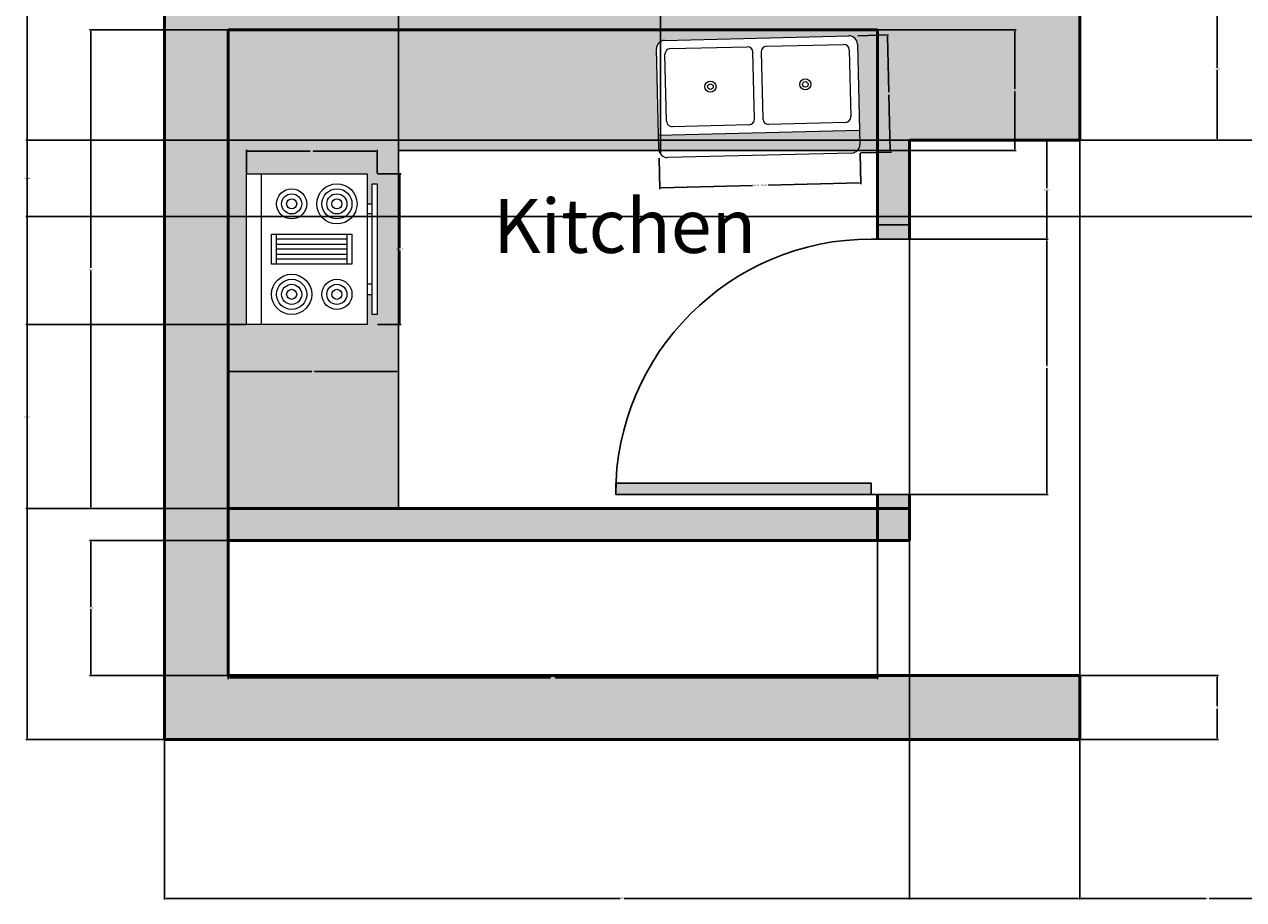
# Model space of a CAD drawing. Units: inches. Extents: x 2578 to 2919, y 51 to 451.
# Tile 1 of 5: x 2578 to 2750, y 51 to 174. Entities that reach past the tile are written whole.
import ezdxf

# ---------------------------------------------------------------- set-up
doc = ezdxf.new("R2010")
doc.units = ezdxf.units.IN
for name, color, linetype, lineweight in [('A-ANNO-DIMS', 2, 'Continuous', 18), ('A-AREA-IDEN', 7, 'Continuous', 25), ('A-DOOR', 4, 'Continuous', 25), ('A-EQPM', 8, 'Continuous', 18), ('A-FLOR-CASE', 8, 'Continuous', 25), ('A-FLOR-FIXT', 9, 'Continuous', 18), ('A-WALL', 7, 'Continuous', 50), ('A-WALL-PATT', 250, 'Continuous', 13)]:
    doc.layers.add(name, color=color, linetype=linetype, lineweight=lineweight)
doc.layers.add('A-CASE-PATT', color=9, linetype='Continuous', lineweight=13, true_color=0xc7c8ca)
doc.layers.add('A-DOOR-PATT', color=29, linetype='Continuous', lineweight=13, true_color=0x4f342a)
doc.styles.get("Standard").update_dxf_attribs({"font": 'arial.ttf'})
doc.dimstyles.get("Standard").update_dxf_attribs({"dimtxt": 0.18, "dimasz": 0.18, "dimexe": 0.18, "dimexo": 0.0625, "dimgap": 0.09, "dimtad": 0, "dimtih": 1, "dimtoh": 1, "dimdec": 4, "dimzin": 0, "dimdsep": 46, "dimtxsty": 'Standard', "dimcen": 0.09, "dimadec": 0, "dimazin": 0, "dimtfac": 1, "dimtdec": 4, "dimtofl": 0, "dimtmove": 0, "dimatfit": 3, "dimfxl": 1, "dimtolj": 1, "dimtzin": 0, "dimarcsym": 0})

# ---------------------------------------------------------------- blocks, each defined once
blk = doc.blocks.new('*U3')
for p, q in [((0, 0), (0, -6)), ((40, 0), (40, -6))]:
    blk.add_line(p, q)
blk.add_lwpolyline([(0, 0), (0, 40), (1.75, 40), (1.75, 0)], close=True)
blk.add_arc((0, 0), 40, 0, 90)
blk = doc.blocks.new('Range-Oven - 30 in top')
for p, q in [((0, -3), (30, -3)), ((12, -6), (18, -6)), ((13, -20), (13, -6)), ((14, -6), (14, -20)), ((15, -20), (15, -6)), ((16, -6), (16, -20)), ((17, -20), (17, -6)), ((18, -20), (12, -20)), ((6, -24), (6, -25)), ((8, -25), (8, -24)), ((22, -25), (22, -24)), ((24, -24), (24, -25))]:
    blk.add_line(p, q)
for points in [[(0, -24), (0, 0), (30, 0), (30, -24)], [(12, -21), (12, -5), (18, -5), (18, -21)], [(2, -26), (2, -25), (28, -25), (28, -26)]]:
    blk.add_lwpolyline(points, close=True)
for centre, radius in [((6, -9), 4), ((6, -9), 3), ((6, -9), 2), ((24, -9), 3), ((24, -9), 2), ((6, -9), 1), ((24, -9), 1), ((24, -18), 4), ((6, -18), 3), ((6, -18), 2), ((24, -18), 3), ((24, -18), 2), ((6, -18), 1), ((24, -18), 1)]:
    blk.add_circle(centre, radius)
blk = doc.blocks.new('Sink-double - 36 in top')
for p, q in [((-18, -4), (18, -4)), ((-0.75, -18.5), (-0.75, -6.5)), ((0.75, -6.5), (0.75, -18.5))]:
    blk.add_line(p, q)
for points in [[(-16.5, 0), (16.5, 0)], [(-18, -19.5), (-18, -1.5)], [(18, -1.5), (18, -19.5)], [(-16.5, -18.5), (-16.5, -6.5)], [(-15.5, -5.5), (-1.75, -5.5)], [(1.75, -5.5), (15.5, -5.5)], [(16.5, -6.5), (16.5, -18.5)], [(-1.75, -19.5), (-15.5, -19.5)], [(15.5, -19.5), (1.75, -19.5)], [(16.5, -21), (-16.5, -21)]]:
    blk.add_lwpolyline(points)
for centre, radius in [((-8.5, -12.5), 1), ((-8.5, -12.5), 0.5), ((8.5, -12.5), 1), ((8.5, -12.5), 0.5)]:
    blk.add_circle(centre, radius)
for centre, radius, start, end in [((-16.5, -1.5), 1.5, 90, 180), ((16.5, -1.5), 1.5, 0, 90), ((-15.5, -6.5), 1, 90, 180), ((-1.75, -6.5), 1, 0, 90), ((1.75, -6.5), 1, 90, 180), ((15.5, -6.5), 1, 0, 90), ((-16.5, -19.5), 1.5, 180, 270), ((-15.5, -18.5), 1, 180, 270), ((-1.75, -18.5), 1, 270, 0), ((1.75, -18.5), 1, 180, 270), ((15.5, -18.5), 1, 270, 0), ((16.5, -19.5), 1.5, 270, 0)]:
    blk.add_arc(centre, radius, start, end)
blk = doc.blocks.new('*D31')
at = {"layer": 'A-ANNO-DIMS', "color": 0, "lineweight": -2, "transparency": 16777216}
for p, q in [((2627.59, 152.86), (2630.9, 152.86)), ((2630.72, 152.68), (2630.72, 142.41)), ((2630.72, 131.78), (2630.72, 142.04)), ((2627.59, 131.6), (2630.9, 131.6))]:
    blk.add_line(p, q, dxfattribs=at)
at = {"layer": 'A-ANNO-DIMS', "color": 0, "transparency": 16777216}
for points in [[(2630.69, 152.68), (2630.75, 152.68), (2630.72, 152.86)], [(2630.69, 131.78), (2630.75, 131.78), (2630.72, 131.6)]]:
    blk.add_solid(points, dxfattribs=at)
at = {"layer": 'Defpoints', "color": 0, "transparency": 16777216}
for p in [(2627.53, 152.86), (2630.72, 152.86), (2627.53, 131.6)]:
    blk.add_point(p, dxfattribs=at)
at = {"layer": 'A-ANNO-DIMS', "color": 0, "transparency": 16777216, "insert": (2630.72, 142.23), "char_height": 0.18, "attachment_point": 5}
blk.add_mtext('\\A1;RANGE 21', dxfattribs=at)
blk = doc.blocks.new('*D32')
at = {"layer": 'A-ANNO-DIMS', "color": 0, "lineweight": -2, "transparency": 16777216}
for p, q in [((2609.1, 152.92), (2609.1, 156.22)), ((2609.28, 156.04), (2618.1, 156.04)), ((2627.35, 156.04), (2618.53, 156.04)), ((2627.53, 152.92), (2627.53, 156.22))]:
    blk.add_line(p, q, dxfattribs=at)
at = {"layer": 'A-ANNO-DIMS', "color": 0, "transparency": 16777216}
for points in [[(2609.28, 156.07), (2609.28, 156.01), (2609.1, 156.04)], [(2627.35, 156.07), (2627.35, 156.01), (2627.53, 156.04)]]:
    blk.add_solid(points, dxfattribs=at)
at = {"layer": 'Defpoints', "color": 0, "transparency": 16777216}
for p in [(2609.1, 156.04), (2609.1, 152.86), (2627.53, 152.86)]:
    blk.add_point(p, dxfattribs=at)
at = {"layer": 'A-ANNO-DIMS', "color": 0, "transparency": 16777216, "insert": (2618.32, 156.04), "char_height": 0.18, "attachment_point": 5}
blk.add_mtext('\\A1;18', dxfattribs=at)
blk = doc.blocks.new('*D33')
at = {"layer": 'A-ANNO-DIMS', "color": 0, "lineweight": -2, "transparency": 16777216}
for p, q in [((2667.26, 155.05), (2667.37, 150.69)), ((2695.58, 155.74), (2695.69, 151.38)), ((2667.54, 150.87), (2680.43, 151.18)), ((2695.5, 151.55), (2682.62, 151.24))]:
    blk.add_line(p, q, dxfattribs=at)
at = {"layer": 'A-ANNO-DIMS', "color": 0, "transparency": 16777216}
for points in [[(2695.5, 151.58), (2695.5, 151.52), (2695.68, 151.56)], [(2667.54, 150.9), (2667.54, 150.84), (2667.36, 150.87)]]:
    blk.add_solid(points, dxfattribs=at)
at = {"layer": 'Defpoints', "color": 0, "transparency": 16777216}
for p in [(2667.26, 155.11), (2695.58, 155.8), (2667.36, 150.87)]:
    blk.add_point(p, dxfattribs=at)
at = {"layer": 'A-ANNO-DIMS', "color": 0, "transparency": 16777216, "insert": (2681.52, 151.21), "char_height": 0.18, "attachment_point": 5}
blk.add_mtext('\\A1;DOUBLE SINK 28', dxfattribs=at)
blk = doc.blocks.new('*D34')
at = {"layer": 'A-ANNO-DIMS', "color": 0, "lineweight": -2, "transparency": 16777216}
for p, q in [((2695.24, 172.32), (2699.6, 172.43)), ((2699.43, 172.25), (2699.62, 164.35)), ((2699.82, 156.09), (2699.63, 163.99)), ((2695.64, 155.8), (2700.01, 155.91))]:
    blk.add_line(p, q, dxfattribs=at)
at = {"layer": 'A-ANNO-DIMS', "color": 0, "transparency": 16777216}
for points in [[(2699.46, 172.25), (2699.4, 172.25), (2699.42, 172.43)], [(2699.85, 156.09), (2699.79, 156.09), (2699.83, 155.91)]]:
    blk.add_solid(points, dxfattribs=at)
at = {"layer": 'Defpoints', "color": 0, "transparency": 16777216}
for p in [(2695.18, 172.32), (2695.58, 155.8), (2699.83, 155.91)]:
    blk.add_point(p, dxfattribs=at)
at = {"layer": 'A-ANNO-DIMS', "color": 0, "transparency": 16777216, "insert": (2699.62, 164.17), "char_height": 0.18, "attachment_point": 5}
blk.add_mtext('\\A1;17', dxfattribs=at)
blk = doc.blocks.new('*D36')
at = {"layer": 'A-ANNO-DIMS', "color": 0, "lineweight": -2, "transparency": 16777216}
for p, q in [((2597.48, 431.14), (2578.02, 431.14)), ((2578.2, 430.96), (2578.2, 252.3)), ((2578.2, 73.28), (2578.2, 251.94)), ((2597.48, 73.1), (2578.02, 73.1))]:
    blk.add_line(p, q, dxfattribs=at)
at = {"layer": 'A-ANNO-DIMS', "color": 0, "transparency": 16777216}
for points in [[(2578.17, 430.96), (2578.23, 430.96), (2578.2, 431.14)], [(2578.17, 73.28), (2578.23, 73.28), (2578.2, 73.1)]]:
    blk.add_solid(points, dxfattribs=at)
at = {"layer": 'Defpoints', "color": 0, "transparency": 16777216}
for p in [(2578.2, 431.14), (2597.55, 431.14), (2597.55, 73.1)]:
    blk.add_point(p, dxfattribs=at)
at = {"layer": 'A-ANNO-DIMS', "color": 0, "transparency": 16777216, "insert": (2578.2, 252.12), "char_height": 0.18, "attachment_point": 5}
blk.add_mtext('\\A1;358.04', dxfattribs=at)
blk = doc.blocks.new('*D43')
at = {"layer": 'A-ANNO-DIMS', "color": 0, "lineweight": -2, "transparency": 16777216}
for p, q in [((2606.48, 173.14), (2587.02, 173.14)), ((2587.2, 172.96), (2587.2, 139.57)), ((2587.2, 105.82), (2587.2, 139.21)), ((2606.48, 105.64), (2587.02, 105.64))]:
    blk.add_line(p, q, dxfattribs=at)
at = {"layer": 'A-ANNO-DIMS', "color": 0, "transparency": 16777216}
for points in [[(2587.17, 172.96), (2587.23, 172.96), (2587.2, 173.14)], [(2587.17, 105.82), (2587.23, 105.82), (2587.2, 105.64)]]:
    blk.add_solid(points, dxfattribs=at)
at = {"layer": 'Defpoints', "color": 0, "transparency": 16777216}
for p in [(2587.2, 173.14), (2606.55, 173.14), (2606.55, 105.64)]:
    blk.add_point(p, dxfattribs=at)
at = {"layer": 'A-ANNO-DIMS', "color": 0, "transparency": 16777216, "insert": (2587.2, 139.39), "char_height": 0.18, "attachment_point": 5}
blk.add_mtext('\\A1;67.5', dxfattribs=at)
blk = doc.blocks.new('*D44')
at = {"layer": 'A-ANNO-DIMS', "color": 0, "lineweight": -2, "transparency": 16777216}
for p, q in [((2606.48, 101.14), (2587.02, 101.14)), ((2587.2, 100.96), (2587.2, 91.8)), ((2587.2, 82.28), (2587.2, 91.44)), ((2606.48, 82.1), (2587.02, 82.1))]:
    blk.add_line(p, q, dxfattribs=at)
at = {"layer": 'A-ANNO-DIMS', "color": 0, "transparency": 16777216}
for points in [[(2587.17, 100.96), (2587.23, 100.96), (2587.2, 101.14)], [(2587.17, 82.28), (2587.23, 82.28), (2587.2, 82.1)]]:
    blk.add_solid(points, dxfattribs=at)
at = {"layer": 'Defpoints', "color": 0, "transparency": 16777216}
for p in [(2587.2, 101.14), (2606.55, 101.14), (2606.55, 82.1)]:
    blk.add_point(p, dxfattribs=at)
at = {"layer": 'A-ANNO-DIMS', "color": 0, "transparency": 16777216, "insert": (2587.2, 91.62), "char_height": 0.18, "attachment_point": 5}
blk.add_mtext('\\A1;19.04', dxfattribs=at)
blk = doc.blocks.new('*D45')
at = {"layer": 'A-ANNO-DIMS', "color": 0, "lineweight": -2, "transparency": 16777216}
for p, q in [((2606.55, 101.08), (2606.55, 81.61)), ((2698.05, 101.08), (2698.05, 81.61)), ((2606.73, 81.79), (2651.97, 81.79)), ((2697.87, 81.79), (2652.62, 81.79))]:
    blk.add_line(p, q, dxfattribs=at)
at = {"layer": 'A-ANNO-DIMS', "color": 0, "transparency": 16777216}
for points in [[(2606.73, 81.82), (2606.73, 81.76), (2606.55, 81.79)], [(2697.87, 81.82), (2697.87, 81.76), (2698.05, 81.79)]]:
    blk.add_solid(points, dxfattribs=at)
at = {"layer": 'Defpoints', "color": 0, "transparency": 16777216}
for p in [(2606.55, 101.14), (2698.05, 101.14), (2606.55, 81.79)]:
    blk.add_point(p, dxfattribs=at)
at = {"layer": 'A-ANNO-DIMS', "color": 0, "transparency": 16777216, "insert": (2652.3, 81.79), "char_height": 0.18, "attachment_point": 5}
blk.add_mtext('\\A1;91.5', dxfattribs=at)
blk = doc.blocks.new('*D50')
at = {"layer": 'A-ANNO-DIMS', "color": 0, "lineweight": -2, "transparency": 16777216}
for p, q in [((2597.55, 73.04), (2597.55, 50.5)), ((2726.55, 73.04), (2726.55, 50.5)), ((2597.73, 50.68), (2661.77, 50.68)), ((2726.37, 50.68), (2662.33, 50.68))]:
    blk.add_line(p, q, dxfattribs=at)
at = {"layer": 'A-ANNO-DIMS', "color": 0, "transparency": 16777216}
for points in [[(2597.73, 50.71), (2597.73, 50.65), (2597.55, 50.68)], [(2726.37, 50.71), (2726.37, 50.65), (2726.55, 50.68)]]:
    blk.add_solid(points, dxfattribs=at)
at = {"layer": 'Defpoints', "color": 0, "transparency": 16777216}
for p in [(2597.55, 73.1), (2726.55, 73.1), (2726.55, 50.68)]:
    blk.add_point(p, dxfattribs=at)
at = {"layer": 'A-ANNO-DIMS', "color": 0, "transparency": 16777216, "insert": (2662.05, 50.68), "char_height": 0.18, "attachment_point": 5}
blk.add_mtext('\\A1;129', dxfattribs=at)
blk = doc.blocks.new('*D51')
at = {"layer": 'A-ANNO-DIMS', "color": 0, "lineweight": -2, "transparency": 16777216}
for p, q in [((2726.55, 73.04), (2726.55, 50.5)), ((2762.55, 73.04), (2762.55, 50.5)), ((2726.73, 50.68), (2744.33, 50.68)), ((2762.37, 50.68), (2744.77, 50.68))]:
    blk.add_line(p, q, dxfattribs=at)
at = {"layer": 'A-ANNO-DIMS', "color": 0, "transparency": 16777216}
for points in [[(2726.73, 50.71), (2726.73, 50.65), (2726.55, 50.68)], [(2762.37, 50.71), (2762.37, 50.65), (2762.55, 50.68)]]:
    blk.add_solid(points, dxfattribs=at)
at = {"layer": 'Defpoints', "color": 0, "transparency": 16777216}
for p in [(2726.55, 73.1), (2762.55, 73.1), (2762.55, 50.68)]:
    blk.add_point(p, dxfattribs=at)
at = {"layer": 'A-ANNO-DIMS', "color": 0, "transparency": 16777216, "insert": (2744.55, 50.68), "char_height": 0.18, "attachment_point": 5}
blk.add_mtext('\\A1;36', dxfattribs=at)
blk = doc.blocks.new('*D56')
at = {"layer": 'A-ANNO-DIMS', "color": 0, "lineweight": -2, "transparency": 16777216}
for p, q in [((2702.61, 143.64), (2722.08, 143.64)), ((2721.9, 143.46), (2721.9, 125.82)), ((2721.9, 107.82), (2721.9, 125.46)), ((2702.61, 107.64), (2722.08, 107.64))]:
    blk.add_line(p, q, dxfattribs=at)
at = {"layer": 'A-ANNO-DIMS', "color": 0, "transparency": 16777216}
for points in [[(2721.87, 143.46), (2721.93, 143.46), (2721.9, 143.64)], [(2721.87, 107.82), (2721.93, 107.82), (2721.9, 107.64)]]:
    blk.add_solid(points, dxfattribs=at)
at = {"layer": 'Defpoints', "color": 0, "transparency": 16777216}
for p in [(2702.55, 143.64), (2702.55, 107.64), (2721.9, 107.64)]:
    blk.add_point(p, dxfattribs=at)
at = {"layer": 'A-ANNO-DIMS', "color": 0, "transparency": 16777216, "insert": (2721.9, 125.64), "char_height": 0.18, "attachment_point": 5}
blk.add_mtext('\\A1;36', dxfattribs=at)
blk = doc.blocks.new('*D59')
at = {"layer": 'A-ANNO-DIMS', "color": 0, "lineweight": -2, "transparency": 16777216}
for p, q in [((2702.61, 157.6), (2722.08, 157.6)), ((2721.9, 157.42), (2721.9, 150.8)), ((2721.9, 143.82), (2721.9, 150.44)), ((2702.61, 143.64), (2722.08, 143.64))]:
    blk.add_line(p, q, dxfattribs=at)
at = {"layer": 'A-ANNO-DIMS', "color": 0, "transparency": 16777216}
for points in [[(2721.87, 157.42), (2721.93, 157.42), (2721.9, 157.6)], [(2721.87, 143.82), (2721.93, 143.82), (2721.9, 143.64)]]:
    blk.add_solid(points, dxfattribs=at)
at = {"layer": 'Defpoints', "color": 0, "transparency": 16777216}
for p in [(2702.55, 157.6), (2702.55, 143.64), (2721.9, 143.64)]:
    blk.add_point(p, dxfattribs=at)
at = {"layer": 'A-ANNO-DIMS', "color": 0, "transparency": 16777216, "insert": (2721.9, 150.62), "char_height": 0.18, "attachment_point": 5}
blk.add_mtext('\\A1;13.958', dxfattribs=at)
blk = doc.blocks.new('*D60')
at = {"layer": 'A-ANNO-DIMS', "color": 0, "lineweight": -2, "transparency": 16777216}
for p, q in [((2726.61, 82.1), (2746.08, 82.1)), ((2745.9, 81.92), (2745.9, 77.78)), ((2745.9, 73.28), (2745.9, 77.42)), ((2726.61, 73.1), (2746.08, 73.1))]:
    blk.add_line(p, q, dxfattribs=at)
at = {"layer": 'A-ANNO-DIMS', "color": 0, "transparency": 16777216}
for points in [[(2745.87, 81.92), (2745.93, 81.92), (2745.9, 82.1)], [(2745.87, 73.28), (2745.93, 73.28), (2745.9, 73.1)]]:
    blk.add_solid(points, dxfattribs=at)
at = {"layer": 'Defpoints', "color": 0, "transparency": 16777216}
for p in [(2726.55, 82.1), (2726.55, 73.1), (2745.9, 73.1)]:
    blk.add_point(p, dxfattribs=at)
at = {"layer": 'A-ANNO-DIMS', "color": 0, "transparency": 16777216, "insert": (2745.9, 77.6), "char_height": 0.18, "attachment_point": 5}
blk.add_mtext('\\A1;9', dxfattribs=at)
blk = doc.blocks.new('*D62')
at = {"layer": 'A-ANNO-DIMS', "color": 0, "lineweight": -2, "transparency": 16777216}
for p, q in [((2606.55, 105.7), (2606.55, 125.17)), ((2606.73, 124.99), (2618.33, 124.99)), ((2630.37, 124.99), (2618.77, 124.99)), ((2630.55, 105.7), (2630.55, 125.17))]:
    blk.add_line(p, q, dxfattribs=at)
at = {"layer": 'A-ANNO-DIMS', "color": 0, "transparency": 16777216}
for points in [[(2606.73, 125.02), (2606.73, 124.96), (2606.55, 124.99)], [(2630.37, 125.02), (2630.37, 124.96), (2630.55, 124.99)]]:
    blk.add_solid(points, dxfattribs=at)
at = {"layer": 'Defpoints', "color": 0, "transparency": 16777216}
for p in [(2630.55, 124.99), (2606.55, 105.64), (2630.55, 105.64)]:
    blk.add_point(p, dxfattribs=at)
at = {"layer": 'A-ANNO-DIMS', "color": 0, "transparency": 16777216, "insert": (2618.55, 124.99), "char_height": 0.18, "attachment_point": 5}
blk.add_mtext('\\A1;24', dxfattribs=at)
blk = doc.blocks.new('*D63')
at = {"layer": 'A-ANNO-DIMS', "color": 0, "lineweight": -2, "transparency": 16777216}
for p, q in [((2698.11, 173.14), (2717.58, 173.14)), ((2717.4, 172.96), (2717.4, 164.82)), ((2717.4, 156.32), (2717.4, 164.46)), ((2698.11, 156.14), (2717.58, 156.14))]:
    blk.add_line(p, q, dxfattribs=at)
at = {"layer": 'A-ANNO-DIMS', "color": 0, "transparency": 16777216}
for points in [[(2717.37, 172.96), (2717.43, 172.96), (2717.4, 173.14)], [(2717.37, 156.32), (2717.43, 156.32), (2717.4, 156.14)]]:
    blk.add_solid(points, dxfattribs=at)
at = {"layer": 'Defpoints', "color": 0, "transparency": 16777216}
for p in [(2698.05, 173.14), (2698.05, 156.14), (2717.4, 156.14)]:
    blk.add_point(p, dxfattribs=at)
at = {"layer": 'A-ANNO-DIMS', "color": 0, "transparency": 16777216, "insert": (2717.4, 164.64), "char_height": 0.18, "attachment_point": 5}
blk.add_mtext('\\A1;17', dxfattribs=at)
blk = doc.blocks.new('*D64')
at = {"layer": 'A-ANNO-DIMS', "color": 0, "lineweight": -2, "transparency": 16777216}
for p, q in [((2702.55, 157.54), (2702.55, 50.5)), ((2726.55, 157.54), (2726.55, 50.5)), ((2702.73, 50.68), (2714.33, 50.68)), ((2726.37, 50.68), (2714.77, 50.68))]:
    blk.add_line(p, q, dxfattribs=at)
at = {"layer": 'A-ANNO-DIMS', "color": 0, "transparency": 16777216}
for points in [[(2702.73, 50.71), (2702.73, 50.65), (2702.55, 50.68)], [(2726.37, 50.71), (2726.37, 50.65), (2726.55, 50.68)]]:
    blk.add_solid(points, dxfattribs=at)
at = {"layer": 'Defpoints', "color": 0, "transparency": 16777216}
for p in [(2702.55, 157.6), (2726.55, 157.6), (2726.55, 50.68)]:
    blk.add_point(p, dxfattribs=at)
at = {"layer": 'A-ANNO-DIMS', "color": 0, "transparency": 16777216, "insert": (2714.55, 50.68), "char_height": 0.18, "attachment_point": 5}
blk.add_mtext('\\A1;24', dxfattribs=at)
blk = doc.blocks.new('*D65')
at = {"layer": 'A-ANNO-DIMS', "color": 0, "lineweight": -2, "transparency": 16777216}
for p, q in [((2726.61, 177.64), (2746.08, 177.64)), ((2745.9, 177.46), (2745.9, 167.8)), ((2745.9, 157.78), (2745.9, 167.44)), ((2726.61, 157.6), (2746.08, 157.6))]:
    blk.add_line(p, q, dxfattribs=at)
at = {"layer": 'A-ANNO-DIMS', "color": 0, "transparency": 16777216}
for points in [[(2745.87, 177.46), (2745.93, 177.46), (2745.9, 177.64)], [(2745.87, 157.78), (2745.93, 157.78), (2745.9, 157.6)]]:
    blk.add_solid(points, dxfattribs=at)
at = {"layer": 'Defpoints', "color": 0, "transparency": 16777216}
for p in [(2726.55, 177.64), (2726.55, 157.6), (2745.9, 157.6)]:
    blk.add_point(p, dxfattribs=at)
at = {"layer": 'A-ANNO-DIMS', "color": 0, "transparency": 16777216, "insert": (2745.9, 167.62), "char_height": 0.18, "attachment_point": 5}
blk.add_mtext('\\A1;20.04', dxfattribs=at)
blk = doc.blocks.new('*D67')
at = {"layer": 'A-ANNO-DIMS', "color": 0, "lineweight": -2, "transparency": 16777216}
for p, q in [((2829.12, 157.6), (2578.02, 157.6)), ((2578.2, 157.42), (2578.2, 152.39)), ((2578.2, 146.99), (2578.2, 152.02)), ((2841.13, 146.81), (2578.02, 146.81))]:
    blk.add_line(p, q, dxfattribs=at)
at = {"layer": 'A-ANNO-DIMS', "color": 0, "transparency": 16777216}
for points in [[(2578.17, 157.42), (2578.23, 157.42), (2578.2, 157.6)], [(2578.17, 146.99), (2578.23, 146.99), (2578.2, 146.81)]]:
    blk.add_solid(points, dxfattribs=at)
at = {"layer": 'Defpoints', "color": 0, "transparency": 16777216}
for p in [(2578.2, 157.6), (2829.18, 157.6), (2841.19, 146.81)]:
    blk.add_point(p, dxfattribs=at)
at = {"layer": 'A-ANNO-DIMS', "color": 0, "transparency": 16777216, "insert": (2578.2, 152.21), "char_height": 0.18, "attachment_point": 5}
blk.add_mtext('\\A1;10.788', dxfattribs=at)
blk = doc.blocks.new('*D69')
at = {"layer": 'A-ANNO-DIMS', "color": 0, "lineweight": -2, "transparency": 16777216}
for p, q in [((2609.04, 131.6), (2578.02, 131.6)), ((2578.2, 131.42), (2578.2, 118.8)), ((2578.2, 105.82), (2578.2, 118.44)), ((2606.48, 105.64), (2578.02, 105.64))]:
    blk.add_line(p, q, dxfattribs=at)
at = {"layer": 'A-ANNO-DIMS', "color": 0, "transparency": 16777216}
for points in [[(2578.17, 131.42), (2578.23, 131.42), (2578.2, 131.6)], [(2578.17, 105.82), (2578.23, 105.82), (2578.2, 105.64)]]:
    blk.add_solid(points, dxfattribs=at)
at = {"layer": 'Defpoints', "color": 0, "transparency": 16777216}
for p in [(2578.2, 131.6), (2609.1, 131.6), (2606.55, 105.64)]:
    blk.add_point(p, dxfattribs=at)
at = {"layer": 'A-ANNO-DIMS', "color": 0, "transparency": 16777216, "insert": (2578.2, 118.62), "char_height": 0.18, "attachment_point": 5}
blk.add_mtext('\\A1;25.955', dxfattribs=at)
blk = doc.blocks.new('*D70')
at = {"layer": 'A-ANNO-DIMS', "color": 0, "lineweight": -2, "transparency": 16777216}
for p, q in [((2630.55, 156.2), (2630.55, 450.67)), ((2630.73, 450.49), (2648.67, 450.49)), ((2667.27, 450.49), (2649.32, 450.49)), ((2667.45, 155.71), (2667.45, 450.67))]:
    blk.add_line(p, q, dxfattribs=at)
at = {"layer": 'A-ANNO-DIMS', "color": 0, "transparency": 16777216}
for points in [[(2630.73, 450.52), (2630.73, 450.46), (2630.55, 450.49)], [(2667.27, 450.52), (2667.27, 450.46), (2667.45, 450.49)]]:
    blk.add_solid(points, dxfattribs=at)
at = {"layer": 'Defpoints', "color": 0, "transparency": 16777216}
for p in [(2667.45, 450.49), (2630.55, 156.14), (2667.45, 155.64)]:
    blk.add_point(p, dxfattribs=at)
at = {"layer": 'A-ANNO-DIMS', "color": 0, "transparency": 16777216, "insert": (2649, 450.49), "char_height": 0.18, "attachment_point": 5}
blk.add_mtext('\\A1;36.9', dxfattribs=at)

msp = doc.modelspace()

# ---------------------------------------------------------------- hatches: boundary and pattern name
at = {"layer": 'A-CASE-PATT'}
h = msp.add_hatch(color=256, dxfattribs=at)
h.dxf.hatch_style = 1
h.paths.add_polyline_path([(2698.047, 173.1406), (2606.547, 173.1406), (2606.547, 105.6406), (2630.547, 105.6406), (2630.547, 156.1406), (2698.047, 156.1406)])
h.paths.add_polyline_path([(2666.8862, 170.4525, -0.41421356), (2668.0374, 171.6612), (2693.9958, 172.2937, -0.41421356), (2695.2045, 171.1425), (2695.5016, 158.9499), (2667.1833, 158.26)], flags=16)
h.paths.add_polyline_path([(2668.0853, 169.6947, -0.41421356), (2668.8528, 170.5005), (2679.6688, 170.764, -0.41421356), (2680.4746, 169.9965), (2680.7046, 160.5571, -0.41421356), (2679.9371, 159.7513), (2669.1211, 159.4878, -0.41421356), (2668.3153, 160.2553)], flags=0)
h.paths.add_polyline_path([(2627.5279, 151.4383), (2627.5279, 133.0127), (2626.8192, 133.0127), (2626.8192, 135.8474), (2626.1105, 135.8474), (2626.1105, 131.5954), (2609.1023, 131.5954), (2609.1023, 152.8557), (2626.1105, 152.8557), (2626.1105, 148.6036), (2626.8192, 148.6036), (2626.8192, 151.4383)], flags=16)
h.paths.add_polyline_path([(2675.2801, 165.1283, -1), (2673.7064, 165.1283, -1)], flags=0)
h.paths.add_polyline_path([(2674.8867, 165.1283, -1), (2674.0999, 165.1283, -1)], flags=0)
h.paths.add_polyline_path([(2624.6932, 148.6036, -1), (2619.0238, 148.6036, -1)], flags=0)
h.paths.add_polyline_path([(2623.9845, 148.6036, -1), (2619.7324, 148.6036, -1)], flags=0)
h.paths.add_polyline_path([(2623.2758, 148.6036, -1), (2620.4411, 148.6036, -1)], flags=0)
h.paths.add_polyline_path([(2622.5671, 148.6036, -1), (2621.1498, 148.6036, -1)], flags=0)
h.paths.add_polyline_path([(2623.9845, 144.3516), (2623.9845, 140.0995), (2612.6457, 140.0995), (2612.6457, 144.3516)], flags=0)
h.paths.add_polyline_path([(2623.2758, 140.8082), (2613.3543, 140.8082), (2613.3543, 143.6429), (2623.2758, 143.6429)], flags=0)
h.paths.add_polyline_path([(2617.6064, 148.6036, -1), (2613.3543, 148.6036, -1)], flags=0)
h.paths.add_polyline_path([(2681.6545, 170.0253, -0.41421356), (2682.422, 170.8311), (2693.238, 171.0946, -0.41421356), (2694.0437, 170.3271), (2694.2737, 160.8877, -0.41421356), (2693.5063, 160.0819), (2682.6903, 159.8184, -0.41421356), (2681.8845, 160.5859)], flags=0)
h.paths.add_polyline_path([(2616.8977, 148.6036, -1), (2614.063, 148.6036, -1)], flags=0)
h.paths.add_polyline_path([(2616.1891, 148.6036, -1), (2614.7717, 148.6036, -1)], flags=0)
h.paths.add_polyline_path([(2623.9845, 135.8474, -1), (2619.7324, 135.8474, -1)], flags=0)
h.paths.add_polyline_path([(2623.2758, 135.8474, -1), (2620.4411, 135.8474, -1)], flags=0)
h.paths.add_polyline_path([(2622.5671, 135.8474, -1), (2621.1498, 135.8474, -1)], flags=0)
h.paths.add_polyline_path([(2688.6526, 165.4541, -1), (2687.0789, 165.4541, -1)], flags=0)
h.paths.add_polyline_path([(2688.2592, 165.4541, -1), (2687.4724, 165.4541, -1)], flags=0)
h.paths.add_polyline_path([(2618.3151, 135.8474, -1), (2612.6457, 135.8474, -1)], flags=0)
h.paths.add_polyline_path([(2617.6064, 135.8474, -1), (2613.3543, 135.8474, -1)], flags=0)
h.paths.add_polyline_path([(2616.8977, 135.8474, -1), (2614.063, 135.8474, -1)], flags=0)
h.paths.add_polyline_path([(2616.1891, 135.8474, -1), (2614.7717, 135.8474, -1)], flags=0)
at = {"layer": 'A-DOOR-PATT'}
h = msp.add_hatch(color=256, dxfattribs=at)
h.dxf.hatch_style = 1
h.paths.add_polyline_path([(2717.5545, 331.5492, 0.01094143), (2715.9791, 331.5147), (2715.9791, 295.5417), (2717.5545, 295.5417)])
h.paths.add_polyline_path([(2772.7563, 343.5147, 0.01094143), (2771.181, 343.5492), (2771.181, 307.5417), (2772.7563, 307.5417)])
h.paths.add_polyline_path([(2809.181, 302.1406), (2807.181, 302.1406), (2807.181, 297.6406), (2809.181, 297.6406)])
h.paths.add_polyline_path([(2681.547, 290.1406), (2679.547, 290.1406), (2679.547, 285.6406), (2681.547, 285.6406)])
h.paths.add_polyline_path([(2870.5896, 193.5988), (2834.5821, 193.5988), (2834.5821, 192.0235), (2870.5551, 192.0235, 0.01094143)])
h.paths.add_polyline_path([(2829.181, 157.5988), (2824.681, 157.5988), (2824.681, 155.5988), (2829.181, 155.5988)])
h.paths.add_polyline_path([(2702.547, 145.6406), (2698.047, 145.6406), (2698.047, 143.6481), (2702.547, 143.6481)])
h.paths.add_polyline_path([(2697.1459, 109.2159), (2661.1384, 109.2159), (2661.1384, 107.6406), (2697.1459, 107.6406)])
h.paths.add_polyline_path([(2702.547, 107.6406), (2698.047, 107.6406), (2698.047, 105.6406), (2702.547, 105.6406)])
h.paths.add_polyline_path([(2771.181, 302.1406), (2769.181, 302.1406), (2769.181, 297.6406), (2771.181, 297.6406)])
at = {"layer": 'A-WALL-PATT'}
h = msp.add_hatch(color=256, dxfattribs=at)
h.dxf.hatch_style = 1
h.paths.add_polyline_path([(2606.547, 422.1406), (2889.181, 422.1406), (2889.181, 210.611), (2824.681, 210.611), (2824.681, 193.5988), (2829.181, 193.5988), (2829.181, 206.111), (2889.181, 206.111), (2889.181, 99.5988), (2829.181, 99.5988), (2829.181, 155.5988), (2824.681, 155.5988), (2824.681, 95.0988), (2889.181, 95.0988), (2889.181, 82.1022), (2762.547, 82.1022), (2762.547, 73.1022), (2898.181, 73.1022), (2898.181, 233.1022), (2898.181, 431.1406), (2597.547, 431.1406), (2597.547, 73.1022), (2726.547, 73.1022), (2726.547, 82.1022), (2606.547, 82.1022), (2606.547, 173.1406), (2698.047, 173.1406), (2698.047, 145.6406), (2702.547, 145.6406), (2702.547, 157.5988), (2726.547, 157.5988), (2726.547, 177.6406), (2606.547, 177.6406)])
h.paths.add_polyline_path([(2889.181, 302.1406), (2809.181, 302.1406), (2809.181, 297.6406), (2889.181, 297.6406)], flags=17)
h.paths.add_polyline_path([(2679.547, 290.1406), (2606.547, 290.1406), (2606.547, 285.6406), (2679.547, 285.6406)], flags=17)
h.paths.add_polyline_path([(2824.681, 157.5988), (2800.681, 157.5988), (2800.681, 155.5988), (2824.681, 155.5988)], flags=17)
h.paths.add_polyline_path([(2698.047, 105.6406), (2606.547, 105.6406), (2606.547, 101.1406), (2698.047, 101.1406)], flags=17)
h.paths.add_polyline_path([(2702.547, 105.6406), (2698.047, 105.6406), (2698.047, 101.1406), (2702.547, 101.1406)], flags=17)
h.paths.add_polyline_path([(2726.547, 422.1406), (2722.047, 422.1406), (2722.047, 295.5417), (2717.5545, 295.5417), (2717.5545, 290.1406), (2717.5504, 285.6406), (2722.047, 285.6406), (2726.547, 285.6406)], flags=17)
h.paths.add_polyline_path([(2769.181, 422.1406), (2764.681, 422.1406), (2764.681, 297.6406), (2769.181, 297.6406)], flags=17)

# ---------------------------------------------------------------- linework, layer by layer
at = {"layer": 'A-DOOR'}
for p, q in [((2698.047, 145.6406), (2702.547, 145.6406)), ((2698.047, 143.6406), (2702.547, 143.6406)), ((2698.047, 107.6406), (2702.547, 107.6406))]:
    msp.add_line(p, q, dxfattribs=at)
at = {"layer": 'A-FLOR-CASE'}
for p, q in [((2630.547, 105.6406), (2630.547, 156.1406)), ((2630.547, 156.1406), (2698.047, 156.1406))]:
    msp.add_line(p, q, dxfattribs=at)
at = {"layer": 'A-WALL'}
for p, q in [((2726.547, 157.5988), (2726.547, 177.6406)), ((2606.547, 82.1022), (2606.547, 173.1406)), ((2606.547, 173.1406), (2698.047, 173.1406)), ((2698.047, 143.6406), (2698.047, 173.1406)), ((2702.547, 143.6406), (2702.547, 157.5988)), ((2726.547, 157.5988), (2702.547, 157.5988)), ((2698.047, 101.1406), (2698.047, 107.6406)), ((2702.547, 101.1406), (2702.547, 107.6406)), ((2606.547, 105.6406), (2702.547, 105.6406)), ((2606.547, 101.1406), (2702.547, 101.1406)), ((2726.547, 82.1022), (2606.547, 82.1022)), ((2726.547, 73.1022), (2726.547, 82.1022))]:
    msp.add_line(p, q, dxfattribs=at)
msp.add_lwpolyline([(2726.547, 73.1022), (2597.547, 73.1022), (2597.547, 431.1406), (2898.181, 431.1406), (2898.181, 233.1022), (2898.181, 73.1022), (2762.547, 73.1022)], dxfattribs=at)

# ---------------------------------------------------------------- block references
at = {"layer": 'A-DOOR', "xscale": 0.9001866182309679, "yscale": 0.9001866182309679, "zscale": 0.9001866182309679, "rotation": 90}
msp.add_blockref('*U3', (2697.1459, 107.6406), dxfattribs=at)
at = {"layer": 'A-EQPM', "xscale": 0.7086762119144434, "yscale": 0.7086762119144434, "zscale": 0.7086762119144434, "rotation": 90}
msp.add_blockref('Range-Oven - 30 in top', (2609.1023, 131.5954), dxfattribs=at)
at = {"layer": 'A-FLOR-FIXT', "xscale": 0.7868516800692607, "yscale": 0.7868516800692607, "zscale": 0.7868516800692607, "rotation": 181.3956621728925}
msp.add_blockref('Sink-double - 36 in top', (2681.4191, 155.4585), dxfattribs=at)

# ---------------------------------------------------------------- texts
at = {"layer": 'A-AREA-IDEN'}
msp.add_text('Kitchen ', height=7.59312, dxfattribs=at).set_placement((2643.8829, 141.6902))

# ---------------------------------------------------------------- dimensions: what is measured, and where the dimension line sits
at = {"layer": 'A-ANNO-DIMS'}
for base, p1, p2, override, picture, middle in [((2667.4454, 450.4906), (2630.547, 156.1406), (2667.4454, 155.6436), {"dimdec": 1, "dimlfac": 1, "dimrnd": 0, "dimzin": 0, "dimdsep": 46, "dimlunit": 2}, '*D70', (2648.9962, 450.4906)), ((2726.547, 50.6838), (2702.547, 157.5988), (2726.547, 157.5988), {"dimdec": 0, "dimlfac": 1, "dimrnd": 0, "dimzin": 0, "dimdsep": 46, "dimlunit": 2}, '*D64', (2714.547, 50.6838)), ((2630.547, 124.9906), (2606.547, 105.6406), (2630.547, 105.6406), {"dimdec": 0, "dimlfac": 1, "dimrnd": 0, "dimzin": 0, "dimdsep": 46, "dimlunit": 2}, '*D62', (2618.547, 124.9906)), ((2726.547, 50.6838), (2597.547, 73.1022), (2726.547, 73.1022), {"dimdec": 0, "dimlfac": 1, "dimrnd": 0, "dimzin": 0, "dimdsep": 46, "dimlunit": 2}, '*D50', (2662.047, 50.6838)), ((2762.547, 50.6838), (2726.547, 73.1022), (2762.547, 73.1022), {"dimdec": 0, "dimlfac": 1, "dimrnd": 0, "dimzin": 0, "dimdsep": 46, "dimlunit": 2}, '*D51', (2744.547, 50.6838))]:
    dim = msp.add_linear_dim(base=base, p1=p1, p2=p2, dimstyle='Standard', override=override, dxfattribs=at)
    dim.commit()
    dim.dimension.update_dxf_attribs({"geometry": picture, "text_midpoint": middle})
for base, p1, p2, angle, override, picture, middle in [((2578.197, 431.1406), (2597.547, 73.1022), (2597.547, 431.1406), 90, {"dimdec": 2, "dimlfac": 1, "dimrnd": 0, "dimzin": 0, "dimdsep": 46, "dimlunit": 2}, '*D36', (2578.197, 252.1214)), ((2745.897, 157.5988), (2726.547, 177.6406), (2726.547, 157.5988), 270, {"dimdec": 2, "dimlfac": 1, "dimrnd": 0, "dimzin": 0, "dimdsep": 46, "dimlunit": 2}, '*D65', (2745.897, 167.6197)), ((2587.197, 173.1406), (2606.547, 105.6406), (2606.547, 173.1406), 90, {"dimdec": 1, "dimlfac": 1, "dimrnd": 0, "dimzin": 0, "dimdsep": 46, "dimlunit": 2}, '*D43', (2587.197, 139.3906)), ((2699.826, 155.9069), (2695.1758, 172.3224), (2695.5782, 155.8034), 271.395662, {"dimdec": 0, "dimlfac": 1, "dimrnd": 0, "dimzin": 0, "dimdsep": 46, "dimlunit": 2}, '*D34', (2699.6247, 164.1664)), ((2717.397, 156.1406), (2698.047, 173.1406), (2698.047, 156.1406), 270, {"dimdec": 0, "dimlfac": 1, "dimrnd": 0, "dimzin": 0, "dimdsep": 46, "dimlunit": 2}, '*D63', (2717.397, 164.6406)), ((2578.197, 157.5988), (2841.1879, 146.8112), (2829.181, 157.5988), 90, {"dimdec": 3, "dimlfac": 1, "dimrnd": 0, "dimzin": 0, "dimdsep": 46, "dimlunit": 2}, '*D67', (2578.197, 152.205)), ((2721.897, 143.6406), (2702.547, 157.5988), (2702.547, 143.6406), 270, {"dimdec": 3, "dimlfac": 1, "dimrnd": 0, "dimzin": 0, "dimdsep": 46, "dimlunit": 2}, '*D59', (2721.897, 150.6197)), ((2609.1023, 156.0447), (2627.5279, 152.8557), (2609.1023, 152.8557), 180, {"dimdec": 0, "dimlfac": 1, "dimrnd": 0, "dimzin": 0, "dimdsep": 46, "dimlunit": 2}, '*D32', (2618.3151, 156.0447)), ((2721.897, 107.6406), (2702.547, 143.6406), (2702.547, 107.6406), 270, {"dimdec": 0, "dimlfac": 1, "dimrnd": 0, "dimzin": 0, "dimdsep": 46, "dimlunit": 2}, '*D56', (2721.897, 125.6406)), ((2578.197, 131.5954), (2606.547, 105.6406), (2609.1023, 131.5954), 90, {"dimdec": 3, "dimlfac": 1, "dimrnd": 0, "dimzin": 0, "dimdsep": 46, "dimlunit": 2}, '*D69', (2578.197, 118.618)), ((2587.197, 101.1406), (2606.547, 82.1022), (2606.547, 101.1406), 90, {"dimdec": 2, "dimlfac": 1, "dimrnd": 0, "dimzin": 0, "dimdsep": 46, "dimlunit": 2}, '*D44', (2587.197, 91.6214)), ((2606.547, 81.7906), (2698.047, 101.1406), (2606.547, 101.1406), 180, {"dimdec": 1, "dimlfac": 1, "dimrnd": 0, "dimzin": 0, "dimdsep": 46, "dimlunit": 2}, '*D45', (2652.297, 81.7906)), ((2745.897, 73.1022), (2726.547, 82.1022), (2726.547, 73.1022), 270, {"dimdec": 0, "dimlfac": 1, "dimrnd": 0, "dimzin": 0, "dimdsep": 46, "dimlunit": 2}, '*D60', (2745.897, 77.6022))]:
    dim = msp.add_linear_dim(base=base, p1=p1, p2=p2, angle=angle, dimstyle='Standard', override=override, dxfattribs=at)
    dim.commit()
    dim.dimension.update_dxf_attribs({"geometry": picture, "text_midpoint": middle})
for base, p1, p2, angle, text, picture, middle in [((2667.3635, 150.8658), (2695.5782, 155.8034), (2667.26, 155.1135), 181.395662, 'DOUBLE SINK <>', '*D33', (2681.5226, 151.2107)), ((2630.7169, 152.8557), (2627.5279, 131.5954), (2627.5279, 152.8557), 90, 'RANGE <>', '*D31', (2630.7169, 142.2255))]:
    dim = msp.add_linear_dim(base=base, p1=p1, p2=p2, angle=angle, text=text, dimstyle='Standard', override={"dimdec": 0, "dimlfac": 1, "dimrnd": 0, "dimzin": 0, "dimdsep": 46, "dimlunit": 2}, dxfattribs=at)
    dim.commit()
    dim.dimension.update_dxf_attribs({"geometry": picture, "text_midpoint": middle})

doc.saveas('drawing.dxf')
